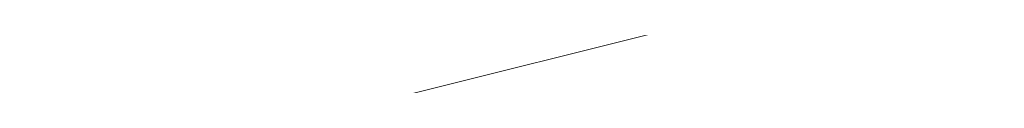
# Model space of a CAD drawing. Units: inches. Extents: x 2091 to 2899, y 967 to 2217.
# Tile 92 of 256: x 2251.2431 to 2251.3854, y 1099.9249 to 1099.9312. Entities that reach past the tile are written whole.
import ezdxf

# ---------------------------------------------------------------- set-up
doc = ezdxf.new("R2010")
doc.units = ezdxf.units.IN
doc.layers.add('A-ANNO-DIMS', color=2, linetype='Continuous', lineweight=18)
doc.layers.add('L-PLNT-TREE', color=94, linetype='Continuous', lineweight=13)
doc.layers.add('A-WALL-PATT', color=141, linetype='Continuous', lineweight=13, true_color=0xadddf7)
doc.styles.get("Standard").update_dxf_attribs({"font": 'arial.ttf'})
doc.dimstyles.new('ISO-25', dxfattribs={"dimtxt": 4, "dimasz": 4, "dimexe": 1.25, "dimexo": 0.625, "dimtad": 1, "dimdec": 0, "dimlunit": 3, "dimtxsty": 'Standard', "dimcen": 2.5, "dimadec": 0, "dimazin": 0, "dimtfac": 1, "dimtdec": 0, "dimtmove": 0, "dimatfit": 3, "dimfxl": 1, "dimarcsym": 0})

# ---------------------------------------------------------------- blocks, each defined once
blk = doc.blocks.new('*U29')
blk.add_line((-402.336, 12.192), (-451.104, 0))
blk = doc.blocks.new('*D71')
at = {"layer": 'A-ANNO-DIMS', "color": 0, "lineweight": -2, "transparency": 16777216}
for p, q in [((2212.1436, 1351.29406), (2212.1436, 969.4643)), ((2452.1436, 1351.29406), (2452.1436, 969.4643)), ((2216.1436, 970.7143), (2448.1436, 970.7143))]:
    blk.add_line(p, q, dxfattribs=at)
at = {"layer": 'A-ANNO-DIMS', "color": 0, "transparency": 16777216}
for points in [[(2216.1436, 971.38097), (2216.1436, 970.04764), (2212.1436, 970.7143)], [(2448.1436, 971.38097), (2448.1436, 970.04764), (2452.1436, 970.7143)]]:
    blk.add_solid(points, dxfattribs=at)
at = {"layer": 'Defpoints', "color": 0, "transparency": 16777216}
for p in [(2212.1436, 1351.91906), (2452.1436, 1351.91906), (2452.1436, 970.7143)]:
    blk.add_point(p, dxfattribs=at)
at = {"layer": 'A-ANNO-DIMS', "color": 0, "transparency": 16777216, "insert": (2332.1436, 973.38159), "char_height": 4, "attachment_point": 5}
blk.add_mtext('20\'-0"', dxfattribs=at)
blk = doc.blocks.new('*D75')
at = {"layer": 'A-ANNO-DIMS', "color": 0, "lineweight": -2, "transparency": 16777216}
for p, q in [((2212.1436, 1274.79406), (2212.1436, 969.4643)), ((2308.1436, 1274.79406), (2308.1436, 969.4643)), ((2216.1436, 970.7143), (2304.1436, 970.7143))]:
    blk.add_line(p, q, dxfattribs=at)
at = {"layer": 'A-ANNO-DIMS', "color": 0, "transparency": 16777216}
for points in [[(2216.1436, 971.38097), (2216.1436, 970.04764), (2212.1436, 970.7143)], [(2304.1436, 971.38097), (2304.1436, 970.04764), (2308.1436, 970.7143)]]:
    blk.add_solid(points, dxfattribs=at)
at = {"layer": 'Defpoints', "color": 0, "transparency": 16777216}
for p in [(2212.1436, 1275.41906), (2308.1436, 1275.41906), (2308.1436, 970.7143)]:
    blk.add_point(p, dxfattribs=at)
at = {"layer": 'A-ANNO-DIMS', "color": 0, "transparency": 16777216, "insert": (2260.1436, 973.38159), "char_height": 4, "attachment_point": 5}
blk.add_mtext('8\'-0"', dxfattribs=at)

msp = doc.modelspace()

# ---------------------------------------------------------------- hatches: boundary and pattern name
at = {"layer": 'A-WALL-PATT'}
h = msp.add_hatch(color=256, dxfattribs=at)
h.dxf.hatch_style = 1
h.paths.add_polyline_path([(2803.1436, 2050.91906), (2203.1436, 2050.91906), (2203.1436, 1090.91906), (2803.1436, 1090.91906)])
h.paths.add_polyline_path([(2635.79885, 1147.54046), (2674.52405, 1147.54046, 0.376086), (2678.52967, 1152.8802), (2678.52967, 1159.55647, 0.333335), (2674.52432, 1163.56185), (2674.52432, 1163.56185), (2674.52432, 1192.93439), (2635.80597, 1192.93439), (2597.08762, 1192.93439), (2597.08762, 1163.56185, 0.333335), (2593.08228, 1159.55647), (2593.08228, 1152.8802, 0.376086), (2597.08789, 1147.54046)], flags=0)
h.paths.add_polyline_path([(2436.01043, 1278.24078, 0.000483), (2435.95264, 1278.21503, -0.001328), (2435.93563, 1278.11169, -0.001711), (2436.11644, 1278.04076, 0.002185)], flags=0)
h.paths.add_polyline_path([(2794.1436, 1143.41906), (2794.1436, 1347.41906), (2543.37017, 1347.41906), (2543.37017, 1351.91906), (2794.1436, 1351.91906), (2794.1436, 1392.71355), (2793.9474, 1392.71355), (2793.9474, 1473.5369), (2794.1436, 1473.5369), (2794.1436, 1531.91906), (2650.1436, 1531.91906), (2650.1436, 1536.41906), (2794.1436, 1536.41906), (2794.1436, 1692.41906), (2609.37561, 1692.41906), (2609.37561, 1644.41906), (2604.87561, 1644.41906), (2604.87561, 1744.91906), (2609.37561, 1744.91906), (2609.37561, 1696.91906), (2794.1436, 1696.91906), (2794.1436, 1780.91906), (2609.6436, 1780.91906), (2493.87561, 1780.91906), (2493.87561, 1785.41906), (2609.6436, 1785.41906), (2794.1436, 1785.41906), (2794.1436, 1847.93882), (2793.95122, 1847.93882), (2793.95122, 1928.76217), (2794.1436, 1928.76217), (2794.1436, 1941.41906), (2614.1436, 1941.41906), (2614.1436, 1821.41906), (2609.6436, 1821.41906), (2609.6436, 1941.41906), (2392.1436, 1941.41906), (2392.1436, 1819.91906), (2387.6436, 1819.91906), (2387.6436, 1941.41906), (2212.1436, 1941.41906), (2212.1436, 1783.91906), (2392.1436, 1783.91906), (2392.1436, 1780.91906), (2212.1436, 1780.91906), (2212.1436, 1629.41906), (2387.6436, 1629.41906), (2387.6436, 1744.91906), (2392.1436, 1744.91906), (2392.1436, 1627.91906), (2317.1436, 1627.91906), (2317.1436, 1551.41906), (2317.1436, 1536.41906), (2459.38359, 1536.41906), (2459.38359, 1602.39648), (2463.88359, 1602.39648), (2463.88359, 1531.91906), (2456.6436, 1531.91906), (2456.6436, 1529.91906), (2452.1436, 1529.91906), (2452.1436, 1531.91906), (2312.6436, 1531.91906), (2312.6436, 1551.41906), (2306.1436, 1551.41906), (2306.1436, 1555.91906), (2308.1436, 1555.91906), (2308.1436, 1551.41906), (2312.6436, 1551.41906), (2312.6436, 1627.91906), (2212.1436, 1627.91906), (2212.1436, 1555.91906), (2270.1436, 1555.91906), (2270.1436, 1551.41906), (2212.1436, 1551.41906), (2212.1436, 1351.91906), (2272.1436, 1351.91906), (2272.1436, 1347.41906), (2212.1436, 1347.41906), (2212.1436, 1275.41906), (2308.1436, 1275.41906), (2308.1436, 1351.91906), (2452.1436, 1351.91906), (2452.1436, 1493.91906), (2456.6436, 1493.91906), (2456.6436, 1347.41906), (2312.6436, 1347.41906), (2312.6436, 1270.91906), (2212.1436, 1270.91906), (2212.1436, 1099.91906), (2281.23752, 1099.91906), (2282.87104, 1110.9138), (2282.00834, 1116.9966), (2278.55774, 1121.4204), (2268.20564, 1128.0562), (2272.08764, 1128.0562), (2273.81294, 1131.927), (2279.42034, 1134.6919), (2285.02784, 1135.2449), (2287.61584, 1137.4568), (2288.04714, 1138.0098), (2289.34114, 1140.7747), (2291.06654, 1139.6687), (2292.36054, 1135.2449), (2295.37984, 1136.9038), (2296.24254, 1135.7979), (2297.10524, 1133.033), (2300.12464, 1138.0098), (2303.14394, 1138.0098), (2304.43794, 1135.7979), (2303.14394, 1133.586), (2306.59464, 1134.6919), (2307.88874, 1133.033), (2310.90804, 1135.2449), (2313.92744, 1134.1389), (2315.62686, 1132.4271), (2308.32004, 1117.5496), (2290.20384, 1109.8079), (2288.90984, 1103.1721), (2289.27231, 1099.91906), (2434.91823, 1099.91906), (2431.59323, 1124.78806), (2429.93023, 1169.55306), (2430.92718, 1240.51969), (2435.65893, 1238.18613), (2437.13523, 1196.55406), (2438.79823, 1143.97306), (2442.67823, 1111.99806), (2446.55823, 1099.91906), (2794.1436, 1099.91906), (2794.1436, 1138.91906), (2548.03245, 1138.91906), (2548.03245, 1143.41906), (2548.03245, 1148.81906), (2546.66846, 1148.03156), (2528.68569, 1179.17862, 0.256256), (2512.03245, 1148.81906), (2512.03245, 1143.41906), (2512.03245, 1138.91906), (2507.53245, 1138.91906), (2507.53245, 1143.41906), (2507.53245, 1148.81906, 0.256256), (2490.8792, 1179.17862), (2472.89644, 1148.03156), (2471.53245, 1148.81906), (2471.53245, 1143.41906), (2467.03245, 1143.41906), (2467.03245, 1269.94579, 0.039061), (2460.90999, 1273.58006), (2467.03245, 1273.58006), (2467.03245, 1286.32536, 0.014511), (2465.21619, 1286.76191), (2467.03245, 1287.05258), (2467.03245, 1323.41906), (2471.53245, 1323.41906), (2471.53245, 1148.81906), (2489.53245, 1179.99597), (2490.89644, 1179.20847), (2490.8792, 1179.17862, -0.256256), (2507.53245, 1148.81906), (2507.53245, 1143.41906), (2512.03245, 1143.41906), (2512.03245, 1148.81906, -0.256256), (2528.68569, 1179.17862), (2528.66846, 1179.20847), (2530.03245, 1179.99597), (2548.03245, 1148.81906), (2548.03245, 1143.41906)], flags=16)
h.paths.add_polyline_path([(2607.76855, 1200.94508), (2607.76855, 1265.03063), (2597.08762, 1281.05201), (2619.78459, 1281.05201), (2627.79528, 1337.12686), (2635.79885, 1337.12686), (2643.81666, 1337.12686), (2651.82736, 1281.05201), (2674.52432, 1281.05201), (2663.8434, 1265.03063), (2663.8434, 1200.94508), (2635.80597, 1200.94508)], flags=0)
edge = h.paths.add_edge_path(flags=0)
edge.add_ellipse((13303.89622, 1272.99872), major_axis=(-10595.31304, 0), ratio=0.84230387009, start_angle=0.628237219, end_angle=0.6465541, ccw=False)
edge.add_ellipse((2711.70045, 1156.85268), major_axis=(2.21977, 0), ratio=0.8423039, start_angle=111.53524, end_angle=180.62824, ccw=False)
edge.add_ellipse((13303.15629, 1272.99872), major_axis=(-10593.02631, 0), ratio=0.84230386954, start_angle=0.528271472, end_angle=0.646554097, ccw=False)
edge.add_line((2710.7646, 1175.3333), (2710.12999, 1175.3333))
edge.add_ellipse((2710.12999, 1176.57978), major_axis=(1.47985, 0), ratio=0.8423039, start_angle=180, end_angle=270, ccw=False)
edge.add_line((2708.65014, 1176.57978), (2708.65014, 1200.78291))
edge.add_ellipse((2710.12999, 1200.78291), major_axis=(1.47985, 0), ratio=0.8423039, start_angle=90, end_angle=180, ccw=False)
edge.add_line((2710.12999, 1202.02939), (2710.46508, 1202.02939))
edge.add_ellipse((13303.15629, 1272.99872), major_axis=(-10593.02631, 0), ratio=0.84230386954, start_angle=-0.090229089, end_angle=0.383866779, ccw=False)
edge.add_ellipse((2710.12999, 1290.92703), major_axis=(-1.47985, 0), ratio=0.8423039, start_angle=0, end_angle=90, ccw=False)
edge.add_line((2708.65014, 1290.92703), (2708.65014, 1315.13017))
edge.add_ellipse((2710.12999, 1315.13017), major_axis=(-1.47985, 0), ratio=0.8423039, start_angle=-90, end_angle=0, ccw=False)
edge.add_line((2710.12999, 1316.37665), (2710.70631, 1316.37665))
edge.add_ellipse((3238.40172, 1296.28957), major_axis=(528.234, 0), ratio=0.84230387, start_angle=176.3495724, end_angle=177.8200497, ccw=False)
edge.add_ellipse((2775.06304, 1071.4507), major_axis=(313.30776, 0), ratio=0.84230387, start_angle=102.1259656, end_angle=103.780529, ccw=False)
edge.add_ellipse((2775.06304, 1078.3057), major_axis=(-305.30289, 0), ratio=0.84230387, start_angle=-79.790461, end_angle=-77.5553727, ccw=False)
edge.add_ellipse((2695.14177, 1541.97538), major_axis=(-250.96022, 0), ratio=0.84230387, start_angle=99.256566, end_angle=102.5549326)
edge.add_line((2741.41033, 1334.21426), (2747.13255, 1337.37848))
edge.add_ellipse((2747.53862, 1336.85748), major_axis=(-0.73992, 0), ratio=0.842304, start_angle=270, end_angle=307.93313, ccw=False)
edge.add_ellipse((2747.53862, 1336.85748), major_axis=(-0.73992, 0), ratio=0.842304, start_angle=232.06687, end_angle=270, ccw=False)
edge.add_line((2747.94469, 1337.37848), (2753.66691, 1334.21426))
edge.add_ellipse((2799.93547, 1541.97538), major_axis=(250.96022, 0), ratio=0.84230387, start_angle=257.4450674, end_angle=260.743434)
edge.add_ellipse((2720.01419, 1078.3057), major_axis=(305.30289, 0), ratio=0.84230387, start_angle=77.5553727, end_angle=79.790461, ccw=False)
edge.add_ellipse((2720.01419, 1071.4507), major_axis=(-313.30776, 0), ratio=0.84230387, start_angle=256.219471, end_angle=257.8740344, ccw=False)
edge.add_ellipse((2256.67551, 1296.28957), major_axis=(-528.234, 0), ratio=0.84230387, start_angle=182.1799503, end_angle=183.6504276, ccw=False)
edge.add_line((2784.37092, 1316.37665), (2784.94725, 1316.37665))
edge.add_ellipse((2784.94725, 1315.13017), major_axis=(1.47985, 0), ratio=0.8423039, start_angle=0, end_angle=90, ccw=False)
edge.add_line((2786.42709, 1315.13017), (2786.42709, 1290.92703))
edge.add_ellipse((2784.94725, 1290.92703), major_axis=(1.47985, 0), ratio=0.8423039, start_angle=270, end_angle=360, ccw=False)
edge.add_ellipse((-7808.07906, 1272.99872), major_axis=(10593.02631, 0), ratio=0.84230386954, start_angle=-0.383866779, end_angle=0.090229089, ccw=False)
edge.add_line((2784.61216, 1202.02939), (2784.94725, 1202.02939))
edge.add_ellipse((2784.94725, 1200.78291), major_axis=(1.47985, 0), ratio=0.8423039, start_angle=0, end_angle=90, ccw=False)
edge.add_line((2786.42709, 1200.78291), (2786.42709, 1176.57978))
edge.add_ellipse((2784.94725, 1176.57978), major_axis=(-1.47985, 0), ratio=0.8423039, start_angle=90, end_angle=180, ccw=False)
edge.add_line((2784.94725, 1175.3333), (2784.31264, 1175.3333))
edge.add_ellipse((-7808.07906, 1272.99872), major_axis=(10593.02631, 0), ratio=0.84230386954, start_angle=-0.618643196, end_angle=-0.528271472, ccw=False)
edge.add_ellipse((2783.37678, 1156.85268), major_axis=(-2.21977, 0), ratio=0.8423039, start_angle=179.37176, end_angle=248.46476, ccw=False)
edge.add_ellipse((-7808.81898, 1272.99872), major_axis=(-10595.31304, 0), ratio=0.84230386576, start_angle=179.353445923, end_angle=179.371762803, ccw=False)
edge.add_ellipse((2780.2973, 1153.50079), major_axis=(-5.24643, 0), ratio=0.8423039, start_angle=90, end_angle=179.35345, ccw=False)
edge.add_line((2780.2973, 1149.08171), (2714.77993, 1149.08171))
edge.add_ellipse((2714.77993, 1153.50079), major_axis=(5.24643, 0), ratio=0.8423039, start_angle=180.64655, end_angle=270, ccw=False)
edge = h.paths.add_edge_path(flags=0)
edge.add_line((2718.18737, 1151.00783), (2718.18737, 1170.47236))
edge.add_ellipse((2721.14706, 1170.47236), major_axis=(-2.95969, 0), ratio=0.8423039, start_angle=-90, end_angle=0, ccw=False)
edge.add_line((2721.14706, 1172.96532), (2773.93017, 1172.96532))
edge.add_ellipse((2773.93017, 1170.47236), major_axis=(-2.95969, 0), ratio=0.8423039, start_angle=180, end_angle=270, ccw=False)
edge.add_line((2776.88987, 1170.47236), (2776.88987, 1151.00783))
edge.add_line((2776.88987, 1151.00783), (2718.18737, 1151.00783))
edge = h.paths.add_edge_path(flags=0)
edge.add_line((2718.18737, 1180.23415), (2718.18737, 1199.05783))
edge.add_ellipse((2747.53862, 1320.39864), major_axis=(147.01792, 0), ratio=0.84230387, start_angle=256.4018653, end_angle=283.5981347)
edge.add_line((2776.88987, 1199.05783), (2776.88987, 1180.23415))
edge.add_ellipse((2747.53862, 1301.57496), major_axis=(147.01792, 0), ratio=0.84230387, start_angle=256.4018653, end_angle=283.5981347, ccw=False)
edge = h.paths.add_edge_path(flags=0)
edge.add_ellipse((13303.15629, 1272.99872), major_axis=(-10591.54646, 0), ratio=0.84230386955, start_angle=0.055594314, end_angle=0.377764194, ccw=False)
edge.add_line((2711.61686, 1262.72171), (2715.66741, 1249.4954))
edge.add_ellipse((6413.89196, 1241.69192), major_axis=(-3698.23616, 0), ratio=0.8423038695, start_angle=-0.12089737, end_angle=0.36407635)
edge.add_line((2715.76104, 1218.19245), (2711.93431, 1203.16736))
edge = h.paths.add_edge_path(flags=0)
edge.add_line((2718.18737, 1251.07457), (2716.00249, 1267.45044))
edge.add_ellipse((2742.15117, 1202.18954), major_axis=(81.77258, 0), ratio=0.84230387, start_angle=94.277421, end_angle=111.8349538, ccw=False)
edge.add_line((2737.00975, 1270.93063), (2758.06748, 1270.93063))
edge.add_ellipse((2752.92606, 1202.18954), major_axis=(81.77258, 0), ratio=0.84230387, start_angle=68.1650462, end_angle=85.722579, ccw=False)
edge.add_line((2779.07475, 1267.45044), (2776.88987, 1251.07457))
edge.add_ellipse((2750.33806, 1187.88536), major_axis=(79.57966, 0), ratio=0.84230387, start_angle=67.2080851, end_angle=85.1299304)
edge.add_line((2756.03466, 1254.74366), (2739.04258, 1254.74366))
edge.add_ellipse((2744.73917, 1187.88536), major_axis=(79.57966, 0), ratio=0.84230387, start_angle=94.8700696, end_angle=112.7919149)
edge = h.paths.add_edge_path(flags=0)
edge.add_line((2783.14293, 1203.16736), (2779.31619, 1218.19245))
edge.add_ellipse((-918.81473, 1241.69192), major_axis=(3698.23616, 0), ratio=0.8423038695, start_angle=-0.36407635, end_angle=0.12089737)
edge.add_line((2779.40983, 1249.4954), (2783.46037, 1262.72171))
edge.add_ellipse((-7808.07906, 1272.99872), major_axis=(-10591.54646, 0), ratio=0.84230386954, start_angle=179.622235806, end_angle=179.944405687, ccw=False)
edge = h.paths.add_edge_path(flags=0)
edge.add_ellipse((2734.20089, 1286.69044), major_axis=(-0.35661, 6.34008), ratio=0.6038336, start_angle=89.002014, end_angle=253.657408, ccw=False)
edge.add_line((2730.369, 1286.54181), (2730.369, 1301.35198))
edge.add_line((2730.369, 1301.35198), (2735.91331, 1305.2148))
edge.add_ellipse((2736.38492, 1304.73456), major_axis=(0.73992, 0), ratio=0.842304, start_angle=90, end_angle=134.48021, ccw=False)
edge.add_line((2736.38492, 1305.3578), (2738.03278, 1305.3578))
edge.add_line((2738.03278, 1305.3578), (2738.03278, 1307.70793))
edge.add_ellipse((2794.20164, 1307.70793), major_axis=(56.16886, 0), ratio=0.84230387, start_angle=150.56143, end_angle=180, ccw=False)
edge.add_ellipse((2700.87559, 1307.70793), major_axis=(-56.16886, 0), ratio=0.84230387, start_angle=180, end_angle=209.43857, ccw=False)
edge.add_line((2757.04445, 1307.70793), (2757.04445, 1305.3578))
edge.add_line((2757.04445, 1305.3578), (2758.69232, 1305.3578))
edge.add_ellipse((2758.69232, 1304.73456), major_axis=(-0.73992, 0), ratio=0.842304, start_angle=225.51979, end_angle=270, ccw=False)
edge.add_line((2759.16392, 1305.2148), (2764.70823, 1301.35198))
edge.add_line((2764.70823, 1301.35198), (2764.70823, 1286.54181))
edge.add_ellipse((2760.87634, 1286.69044), major_axis=(0.35661, 6.34008), ratio=0.6038336, start_angle=106.342592, end_angle=270.997986, ccw=False)
edge.add_line((2757.04445, 1285.79709), (2757.04445, 1307.70793))
edge.add_ellipse((2700.87559, 1307.70793), major_axis=(-56.16886, 0), ratio=0.84230387, start_angle=180, end_angle=209.43857)
edge.add_ellipse((2794.20164, 1307.70793), major_axis=(56.16886, 0), ratio=0.84230387, start_angle=150.56143, end_angle=180)
edge.add_line((2738.03278, 1307.70793), (2738.03278, 1285.79709))
h.paths.add_polyline_path([(2417.81227, 1104.4497), (2413.49227, 1102.5297), (2410.61227, 1103.9697), (2409.17227, 1106.3697), (2407.25227, 1107.3297), (2406.29227, 1109.7297), (2405.33227, 1114.0497), (2405.33227, 1117.8897), (2406.29227, 1120.1297), (2407.25227, 1119.8097), (2408.84832, 1118.32766), (2410.17395, 1119.42417), (2410.21127, 1120.4057), (2411.04073, 1121.41905), (2410.69927, 1119.8587), (2410.17395, 1119.42417), (2410.08845, 1117.17611), (2411.13284, 1116.20632), (2413.97227, 1119.3297), (2416.85227, 1120.7697), (2416.86972, 1120.79878), (2417.03507, 1119.40512), (2417.89621, 1118.14338), (2418.29227, 1118.3697), (2419.54445, 1120.03927), (2419.36092, 1118.38749), (2419.03211, 1119.35615), (2418.39894, 1118.51193), (2419.25227, 1114.5297), (2418.79409, 1107.19879)], flags=0)
h.paths.add_polyline_path([(2508.87017, 1347.41906), (2508.37017, 1347.41906), (2508.37017, 1351.91906), (2508.87017, 1351.91906)], flags=0)
h.paths.add_polyline_path([(2473.37017, 1347.41906), (2472.37017, 1347.41906), (2467.87017, 1347.41906), (2467.87017, 1455.41906), (2472.37017, 1455.41906), (2472.37017, 1352.41906), (2473.37017, 1352.41906)], flags=0)
h.paths.add_polyline_path([(2352.10624, 1217.4462), (2349.22624, 1218.8862), (2347.78624, 1221.2862), (2345.86624, 1222.2462), (2344.90624, 1224.6462), (2343.94624, 1228.9662), (2343.94624, 1232.8062), (2344.90624, 1235.0462), (2345.86624, 1234.7262), (2347.46229, 1233.24415), (2348.78792, 1234.34066), (2348.82524, 1235.3222), (2349.6547, 1236.33555), (2349.31324, 1234.7752), (2348.78792, 1234.34066), (2348.70242, 1232.0926), (2349.74681, 1231.12282), (2352.58624, 1234.2462), (2355.46624, 1235.6862), (2355.48369, 1235.71528), (2355.64904, 1234.32161), (2356.51018, 1233.05988), (2356.90624, 1233.2862), (2358.15842, 1234.95576), (2357.97489, 1233.30398), (2357.64608, 1234.27264), (2357.01291, 1233.42842), (2357.86624, 1229.4462), (2357.40806, 1222.11529), (2356.42624, 1219.3662)], flags=0)
h.paths.add_polyline_path([(2348.2968, 1112.22442), (2347.0138, 1112.31042), (2345.5298, 1114.12742), (2345.7318, 1115.85842), (2346.8118, 1116.98242), (2346.8118, 1114.64642), (2345.8668, 1114.21442), (2346.8798, 1114.30042)], flags=0)
h.paths.add_polyline_path([(2347.0138, 1110.92642), (2346.2718, 1110.49342), (2346.6098, 1111.18642)], flags=0)
h.paths.add_polyline_path([(2345.8668, 1118.19442), (2345.5298, 1117.32942), (2343.7078, 1118.02142), (2344.3828, 1118.62642)], flags=0)
h.paths.add_polyline_path([(2346.6768, 1109.28242), (2346.0698, 1108.07142), (2345.8668, 1110.06142)], flags=0)
h.paths.add_polyline_path([(2345.0568, 1119.75142), (2343.6398, 1119.75142), (2343.9778, 1121.13542)], flags=0)
h.paths.add_polyline_path([(2345.2598, 1116.55042), (2345.1248, 1115.85842), (2344.9218, 1115.68542), (2344.7198, 1116.37742)], flags=0)
h.paths.add_polyline_path([(2345.6648, 1112.31042), (2345.4618, 1111.53242), (2344.0448, 1111.96442), (2344.6518, 1112.57042)], flags=0)
h.paths.add_polyline_path([(2345.1918, 1113.34942), (2344.4498, 1113.86842), (2344.7198, 1114.38742)], flags=0)
h.paths.add_polyline_path([(2344.6518, 1116.80942), (2344.1798, 1115.68542), (2344.6518, 1115.33942), (2343.9098, 1114.90642), (2343.0328, 1115.94442), (2343.6398, 1116.46342)], flags=0)
h.paths.add_polyline_path([(2345.8668, 1106.68642), (2344.9898, 1105.56242), (2344.5168, 1106.60042)], flags=0)
h.paths.add_polyline_path([(2344.8548, 1110.06142), (2344.5168, 1109.28242), (2344.1128, 1109.71542)], flags=0)
h.paths.add_polyline_path([(2344.0448, 1113.52242), (2343.4378, 1113.08942), (2342.7628, 1113.95442)], flags=0)
h.paths.add_polyline_path([(2344.3148, 1111.01242), (2342.9648, 1110.32042), (2342.9648, 1111.09942)], flags=0)
h.paths.add_polyline_path([(2345.1248, 1104.69742), (2344.5848, 1103.74542), (2344.4498, 1104.26442)], flags=0)
h.paths.add_polyline_path([(2342.8298, 1121.22242), (2341.7498, 1120.53042), (2340.5358, 1121.04942), (2340.1308, 1121.82842), (2340.6708, 1122.95242), (2341.1428, 1121.82842), (2341.6148, 1122.00142)], flags=0)
h.paths.add_polyline_path([(2342.9648, 1119.75142), (2343.0328, 1118.45342), (2342.0878, 1118.02142), (2342.0198, 1119.49142)], flags=0)
h.paths.add_polyline_path([(2342.6948, 1116.89642), (2341.9528, 1116.63642), (2342.0198, 1117.32942)], flags=0)
h.paths.add_polyline_path([(2343.0328, 1112.22442), (2342.0198, 1111.79142), (2341.5478, 1112.22442), (2342.3578, 1113.34942)], flags=0)
h.paths.add_polyline_path([(2343.7748, 1104.43742), (2342.6278, 1102.88042), (2342.6948, 1104.61042), (2343.4378, 1105.12942)], flags=0)
h.paths.add_polyline_path([(2342.0198, 1115.07942), (2340.8058, 1115.51242), (2340.9408, 1116.37742)], flags=0)
h.paths.add_polyline_path([(2341.4808, 1120.09742), (2341.4808, 1119.40542), (2341.0758, 1119.57842), (2341.1428, 1120.09742)], flags=0)
h.paths.add_polyline_path([(2341.8178, 1114.47342), (2340.9408, 1113.08942), (2340.8058, 1114.56042)], flags=0)
h.paths.add_polyline_path([(2341.1428, 1118.54042), (2340.9408, 1116.98242), (2339.0508, 1117.67542), (2339.0508, 1118.62642)], flags=0)
h.paths.add_polyline_path([(2342.6948, 1101.66842), (2341.9528, 1101.84142), (2342.5598, 1102.36142)], flags=0)
h.paths.add_polyline_path([(2340.3328, 1119.66542), (2338.4438, 1119.57842), (2337.9038, 1120.35742), (2339.6578, 1120.61642)], flags=0)
h.paths.add_polyline_path([(2340.3328, 1115.33942), (2340.0628, 1113.69542), (2339.3878, 1115.33942)], flags=0)
h.paths.add_polyline_path([(2341.8178, 1103.83142), (2341.5478, 1102.88042), (2341.1428, 1103.65842)], flags=0)
h.paths.add_polyline_path([(2339.0508, 1122.86642), (2337.2958, 1121.82842), (2337.0938, 1123.12542), (2337.7688, 1123.81842)], flags=0)
h.paths.add_polyline_path([(2339.1178, 1121.74142), (2338.8478, 1121.22242), (2338.1738, 1121.04942), (2338.3758, 1121.56842)], flags=0)
h.paths.add_polyline_path([(2339.1858, 1119.31942), (2338.6458, 1118.71342), (2338.2408, 1118.10742), (2338.2408, 1118.88642)], flags=0)
h.paths.add_polyline_path([(2341.1428, 1101.92842), (2340.6028, 1101.23642), (2340.0628, 1101.84142), (2340.6028, 1102.36142)], flags=0)
h.paths.add_polyline_path([(2337.6338, 1117.76142), (2336.6208, 1118.28042), (2337.2958, 1118.97242)], flags=0)
h.paths.add_polyline_path([(2336.8238, 1119.57842), (2334.7988, 1118.97242), (2335.2038, 1120.35742), (2336.5538, 1120.87642)], flags=0)
h.paths.add_polyline_path([(2339.1178, 1100.45742), (2337.3638, 1100.54342), (2336.7558, 1101.23642)], flags=0)
h.paths.add_polyline_path([(2336.3508, 1122.43342), (2336.0138, 1121.91442), (2334.9338, 1122.43342), (2334.5288, 1123.47142), (2335.7438, 1122.77942)], flags=0)
h.paths.add_polyline_path([(2334.7318, 1120.87642), (2334.2588, 1120.35742), (2334.0568, 1120.78942), (2334.5968, 1121.30842)], flags=0)
h.paths.add_polyline_path([(2334.4618, 1122.17442), (2332.5718, 1121.30842), (2331.3568, 1122.17442), (2332.0998, 1122.86642)], flags=0)
h.paths.add_polyline_path([(2334.2588, 1118.54042), (2333.3818, 1118.45342), (2333.6518, 1119.31942)], flags=0)
h.paths.add_polyline_path([(2335.5418, 1102.27442), (2334.1918, 1102.62042), (2335.2718, 1103.31242)], flags=0)
h.paths.add_polyline_path([(2332.7068, 1119.66542), (2331.6948, 1120.44342), (2332.5048, 1120.78942)], flags=0)
h.paths.add_polyline_path([(2334.7318, 1101.14942), (2333.5168, 1101.58242), (2333.9888, 1101.75542)], flags=0)
h.paths.add_polyline_path([(2332.6398, 1116.63642), (2331.0868, 1116.29042), (2331.9648, 1118.19442)], flags=0)
h.paths.add_polyline_path([(2330.7498, 1121.56842), (2330.2768, 1120.27042), (2328.5228, 1119.31942), (2328.9948, 1121.04942)], flags=0)
h.paths.add_polyline_path([(2330.7498, 1118.62642), (2330.0078, 1117.50242), (2329.8728, 1118.02142)], flags=0)
h.paths.add_polyline_path([(2332.0998, 1102.36142), (2330.5468, 1102.01442), (2331.6948, 1102.96642)], flags=0)
h.paths.add_polyline_path([(2329.5348, 1113.60842), (2329.0628, 1112.31042), (2328.5898, 1113.34942)], flags=0)
h.paths.add_polyline_path([(2328.3878, 1117.84842), (2327.5098, 1116.55042), (2327.1728, 1117.76142)], flags=0)
h.paths.add_polyline_path([(2329.7378, 1106.51342), (2329.5348, 1105.30242), (2328.2528, 1106.08142)], flags=0)
h.paths.add_polyline_path([(2328.6578, 1114.38742), (2328.0498, 1114.12742), (2328.3198, 1114.90642)], flags=0)
h.paths.add_polyline_path([(2328.3198, 1112.22442), (2327.1058, 1112.13742), (2326.7008, 1112.65642)], flags=0)
h.paths.add_polyline_path([(2326.9028, 1115.25242), (2326.7008, 1114.12742), (2325.2158, 1113.60842), (2326.0928, 1115.33942)], flags=0)
h.paths.add_polyline_path([(2326.6328, 1108.33042), (2326.0928, 1107.37942), (2325.8908, 1108.50342), (2326.4978, 1109.10942)], flags=0)
h.paths.add_polyline_path([(2615.1436, 1531.91906), (2609.6436, 1531.91906), (2609.6436, 1620.41906), (2614.1436, 1620.41906), (2614.1436, 1536.41906), (2615.1436, 1536.41906)], flags=0)
h.paths.add_polyline_path([(2545.1436, 1563.41906), (2464.1436, 1563.41906), (2464.1436, 1632.41906), (2509.1436, 1632.41906), (2509.1436, 1627.91906), (2509.1436, 1603.91906), (2468.6436, 1603.91906), (2468.6436, 1567.91906), (2540.6436, 1567.91906), (2540.6436, 1591.91906), (2545.1436, 1591.91906)], flags=0)
h.paths.add_polyline_path([(2388.96905, 1549.98573), (2357.43418, 1549.98573), (2357.43418, 1623.36078), (2399.36278, 1623.36078), (2435.68947, 1623.36078), (2435.59255, 1602.55927), (2435.59255, 1602.39648), (2388.96905, 1602.39648)], flags=0)
h.paths.add_polyline_path([(2388.88063, 1555.80915), (2374.90443, 1555.80915), (2374.90443, 1600.57156), (2374.90443, 1615.45765), (2406.35088, 1615.45765), (2406.35088, 1618.93943), (2412.17429, 1615.45765), (2406.35088, 1611.97586), (2406.35088, 1615.45765), (2388.88063, 1615.45765)], flags=0)
h.paths.add_polyline_path([(2568.87561, 1644.41906), (2453.37561, 1644.41906), (2453.37561, 1785.41906), (2457.87561, 1785.41906), (2457.87561, 1648.91906), (2568.87561, 1648.91906)], flags=0)
h.paths.add_polyline_path([(2212.1436, 1945.91906), (2212.1436, 2041.91906), (2794.1436, 2041.91906), (2794.1436, 1945.91906)], flags=16)
h.paths.add_polyline_path([(2271.08273, 1964.31724), (2776.85297, 1964.31724), (2776.85297, 2037.16962), (2271.08273, 2037.16962)], flags=8)
h.paths.add_polyline_path([(2380.64929, 1536.82414), (2461.04081, 1536.82414), (2461.04081, 1554.65259), (2380.64929, 1554.65259)], flags=8)
h.paths.add_polyline_path([(2240.75571, 1609.72545), (2309.18583, 1609.72545), (2309.18583, 1617.6982), (2240.75571, 1617.6982)], flags=8)
h.paths.add_polyline_path([(2212.67726, 1313.5041), (2282.59152, 1313.5041), (2282.59152, 1322.74524), (2212.67726, 1322.74524)], flags=8)
h.paths.add_polyline_path([(2457.11198, 1114.77857), (2558.48158, 1114.77857), (2558.48158, 1142.21968), (2457.11198, 1142.21968)], flags=8)
h.paths.add_polyline_path([(2473.44234, 1273.01007), (2604.64123, 1273.01007), (2604.64123, 1318.34693), (2473.44234, 1318.34693)], flags=8)
h.paths.add_polyline_path([(2638.8763, 1626.97743), (2684.25037, 1627.97674), (2684.03848, 1637.59749), (2638.66442, 1636.59819)], flags=8)
h.paths.add_polyline_path([(2537.59055, 1453.79345), (2628.38955, 1453.79345), (2628.38955, 1475.34481), (2537.59055, 1475.34481)], flags=8)
h.paths.add_polyline_path([(2504.13764, 1714.6324), (2554.64719, 1714.6324), (2554.64719, 1730.23771), (2504.13764, 1730.23771)], flags=8)
h.paths.add_polyline_path([(2487.50118, 1575.65187), (2535.09712, 1575.65187), (2535.09712, 1598.37765), (2487.50118, 1598.37765)], flags=8)
h.paths.add_polyline_path([(2709.0994, 1735.71028), (2740.0166, 1735.71028), (2740.0166, 1749.93764), (2709.0994, 1749.93764)], flags=8)
h.paths.add_polyline_path([(2442.43842, 1792.17166), (2564.72884, 1792.17166), (2564.72884, 1842.00016), (2442.43842, 1842.00016)], flags=8)
h.paths.add_polyline_path([(2655.8158, 1809.64408), (2789.52014, 1806.6938), (2790.08498, 1832.29164), (2656.38064, 1835.24192)], flags=8)
h.paths.add_polyline_path([(2234.8427, 1797.72014), (2368.59285, 1794.76885), (2369.16072, 1820.50413), (2235.41056, 1823.45542)], flags=8)
h.paths.add_polyline_path([(2245.13847, 1644.00633), (2398.42773, 1640.6239), (2398.99484, 1666.32482), (2245.70557, 1669.70725)], flags=8)
h.paths.add_polyline_path([(2306.14285, 1431.16852), (2413.76831, 1428.79369), (2414.33315, 1454.39153), (2306.70768, 1456.76636)], flags=8)
h.paths.add_polyline_path([(2306.83458, 1458.23314), (2393.38048, 1456.32345), (2393.93281, 1481.35436), (2307.38691, 1483.26405)], flags=8)

# ---------------------------------------------------------------- block references
at = {"layer": 'L-PLNT-TREE', "xscale": 0.0393700787401575, "yscale": 0.0393700787401575, "zscale": 0.0393700787401575}
msp.add_blockref('*U29', (2269.04101, 1099.91906), dxfattribs=at)

# ---------------------------------------------------------------- dimensions: what is measured, and where the dimension line sits
at = {"layer": 'A-ANNO-DIMS'}
for base, p1, p2, picture, middle in [((2452.1436, 970.7143), (2212.1436, 1351.91906), (2452.1436, 1351.91906), '*D71', (2332.1436, 973.38159)), ((2308.1436, 970.7143), (2212.1436, 1275.41906), (2308.1436, 1275.41906), '*D75', (2260.1436, 973.38159))]:
    dim = msp.add_linear_dim(base=base, p1=p1, p2=p2, dimstyle='ISO-25', override={"dimdec": 1, "dimlfac": 1, "dimrnd": 0, "dimzin": 1, "dimdsep": 46, "dimlunit": 4, "dimfrac": 2}, dxfattribs=at)
    dim.commit()
    dim.dimension.update_dxf_attribs({"geometry": picture, "text_midpoint": middle})

doc.saveas('drawing.dxf')
